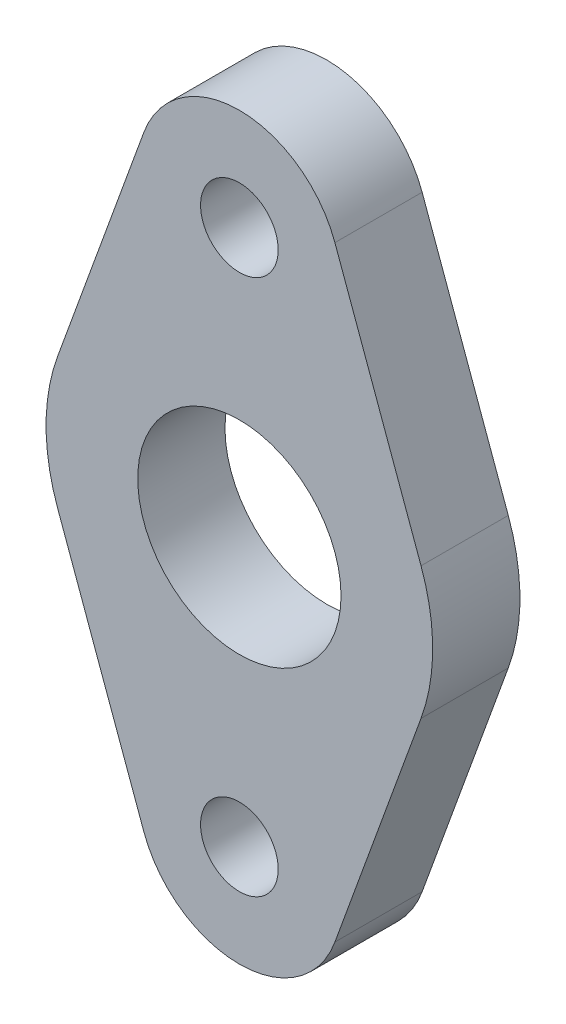
ISO-10303-21;
HEADER;
FILE_DESCRIPTION(('STEP AP214'),'2;1');
FILE_NAME('part.step','',(''),(''),'','','');
FILE_SCHEMA(('AUTOMOTIVE_DESIGN { 1 0 10303 214 1 1 1 1 }'));
ENDSEC;
DATA;
#1=APPLICATION_CONTEXT('core data for automotive mechanical design processes');
#2=APPLICATION_PROTOCOL_DEFINITION('international standard','automotive_design',2000,#1);
#3=PRODUCT_CONTEXT('',#1,'mechanical');
#4=PRODUCT('Part','Part','',(#3));
#5=PRODUCT_RELATED_PRODUCT_CATEGORY('part','',(#4));
#6=PRODUCT_DEFINITION_FORMATION('','',#4);
#7=PRODUCT_DEFINITION_CONTEXT('part definition',#1,'design');
#8=PRODUCT_DEFINITION('design','',#6,#7);
#9=PRODUCT_DEFINITION_SHAPE('','',#8);
#10=(LENGTH_UNIT() NAMED_UNIT(*) SI_UNIT(.MILLI.,.METRE.));
#11=(NAMED_UNIT(*) PLANE_ANGLE_UNIT() SI_UNIT($,.RADIAN.));
#12=(NAMED_UNIT(*) SI_UNIT($,.STERADIAN.) SOLID_ANGLE_UNIT());
#13=UNCERTAINTY_MEASURE_WITH_UNIT(LENGTH_MEASURE(1.E-05),#10,'distance_accuracy_value','');
#14=(GEOMETRIC_REPRESENTATION_CONTEXT(3) GLOBAL_UNCERTAINTY_ASSIGNED_CONTEXT((#13)) GLOBAL_UNIT_ASSIGNED_CONTEXT((#10,
#11,#12)) REPRESENTATION_CONTEXT('',''));
#15=CARTESIAN_POINT('',(0.,0.,0.));
#16=DIRECTION('',(0.,0.,1.));
#17=DIRECTION('',(1.,0.,0.));
#18=AXIS2_PLACEMENT_3D('',#15,#16,#17);
#19=CARTESIAN_POINT('',(0.,-33.5,10.9));
#20=DIRECTION('',(0.,0.,-1.));
#21=DIRECTION('',(-1.,0.,0.));
#22=AXIS2_PLACEMENT_3D('',#19,#20,#21);
#23=CYLINDRICAL_SURFACE('',#22,12.7);
#24=CARTESIAN_POINT('',(0.,-33.5,0.));
#25=DIRECTION('',(0.,0.,1.));
#26=DIRECTION('',(-1.,0.,0.));
#27=AXIS2_PLACEMENT_3D('',#24,#25,#26);
#28=CIRCLE('',#27,12.7);
#29=CARTESIAN_POINT('',(-11.9351548725244,-37.8407462686567,0.));
#30=VERTEX_POINT('',#29);
#31=CARTESIAN_POINT('',(11.9351548725244,-37.8407462686567,0.));
#32=VERTEX_POINT('',#31);
#33=EDGE_CURVE('E140',#30,#32,#28,.T.);
#34=ORIENTED_EDGE('',*,*,#33,.T.);
#35=DIRECTION('',(0.,0.,-1.));
#36=VECTOR('',#35,1.);
#37=CARTESIAN_POINT('',(11.9351548725244,-37.8407462686567,10.9));
#38=LINE('',#37,#36);
#39=CARTESIAN_POINT('',(11.9351548725244,-37.8407462686567,10.9));
#40=VERTEX_POINT('',#39);
#41=EDGE_CURVE('E11',#40,#32,#38,.T.);
#42=ORIENTED_EDGE('',*,*,#41,.F.);
#43=CARTESIAN_POINT('',(0.,-33.5,10.9));
#44=DIRECTION('',(0.,0.,1.));
#45=DIRECTION('',(-1.,0.,0.));
#46=AXIS2_PLACEMENT_3D('',#43,#44,#45);
#47=CIRCLE('',#46,12.7);
#48=CARTESIAN_POINT('',(-11.9351548725244,-37.8407462686567,10.9));
#49=VERTEX_POINT('',#48);
#50=EDGE_CURVE('E151',#49,#40,#47,.T.);
#51=ORIENTED_EDGE('',*,*,#50,.F.);
#52=DIRECTION('',(0.,0.,-1.));
#53=VECTOR('',#52,1.);
#54=CARTESIAN_POINT('',(-11.9351548725244,-37.8407462686567,10.9));
#55=LINE('',#54,#53);
#56=EDGE_CURVE('E135',#49,#30,#55,.T.);
#57=ORIENTED_EDGE('',*,*,#56,.T.);
#58=EDGE_LOOP('',(#34,#42,#51,#57));
#59=FACE_BOUND('',#58,.T.);
#60=ADVANCED_FACE('F39',(#59),#23,.T.);
#61=CARTESIAN_POINT('',(11.9351548725244,-37.8407462686567,10.9));
#62=DIRECTION('',(-0.939775974214519,0.341791044776119,0.));
#63=DIRECTION('',(-0.341791044776119,-0.939775974214519,0.));
#64=AXIS2_PLACEMENT_3D('',#61,#62,#63);
#65=PLANE('',#64);
#66=DIRECTION('',(0.341791044776119,0.939775974214519,0.));
#67=VECTOR('',#66,1.);
#68=CARTESIAN_POINT('',(11.9351548725244,-37.8407462686567,0.));
#69=LINE('',#68,#67);
#70=CARTESIAN_POINT('',(22.6955897772806,-8.25425373134328,0.));
#71=VERTEX_POINT('',#70);
#72=EDGE_CURVE('E139',#32,#71,#69,.T.);
#73=ORIENTED_EDGE('',*,*,#72,.T.);
#74=DIRECTION('',(0.,0.,-1.));
#75=VECTOR('',#74,1.);
#76=CARTESIAN_POINT('',(22.6955897772806,-8.25425373134328,10.9));
#77=LINE('',#76,#75);
#78=CARTESIAN_POINT('',(22.6955897772806,-8.25425373134328,10.9));
#79=VERTEX_POINT('',#78);
#80=EDGE_CURVE('E48',#79,#71,#77,.T.);
#81=ORIENTED_EDGE('',*,*,#80,.F.);
#82=DIRECTION('',(0.341791044776119,0.939775974214519,0.));
#83=VECTOR('',#82,1.);
#84=CARTESIAN_POINT('',(11.9351548725244,-37.8407462686567,10.9));
#85=LINE('',#84,#83);
#86=EDGE_CURVE('E99',#40,#79,#85,.T.);
#87=ORIENTED_EDGE('',*,*,#86,.F.);
#88=ORIENTED_EDGE('',*,*,#41,.T.);
#89=EDGE_LOOP('',(#73,#81,#87,#88));
#90=FACE_BOUND('',#89,.T.);
#91=ADVANCED_FACE('F199',(#90),#65,.F.);
#92=CARTESIAN_POINT('',(0.,0.,10.9));
#93=DIRECTION('',(0.,0.,-1.));
#94=DIRECTION('',(-1.,0.,0.));
#95=AXIS2_PLACEMENT_3D('',#92,#93,#94);
#96=CYLINDRICAL_SURFACE('',#95,24.15);
#97=CARTESIAN_POINT('',(0.,0.,0.));
#98=DIRECTION('',(0.,0.,1.));
#99=DIRECTION('',(1.,0.,0.));
#100=AXIS2_PLACEMENT_3D('',#97,#98,#99);
#101=CIRCLE('',#100,24.15);
#102=CARTESIAN_POINT('',(22.6955897772806,8.25425373134328,0.));
#103=VERTEX_POINT('',#102);
#104=EDGE_CURVE('E142',#71,#103,#101,.T.);
#105=ORIENTED_EDGE('',*,*,#104,.T.);
#106=DIRECTION('',(0.,0.,-1.));
#107=VECTOR('',#106,1.);
#108=CARTESIAN_POINT('',(22.6955897772806,8.25425373134328,10.9));
#109=LINE('',#108,#107);
#110=CARTESIAN_POINT('',(22.6955897772806,8.25425373134328,10.9));
#111=VERTEX_POINT('',#110);
#112=EDGE_CURVE('E158',#111,#103,#109,.T.);
#113=ORIENTED_EDGE('',*,*,#112,.F.);
#114=CARTESIAN_POINT('',(0.,0.,10.9));
#115=DIRECTION('',(0.,0.,1.));
#116=DIRECTION('',(1.,0.,0.));
#117=AXIS2_PLACEMENT_3D('',#114,#115,#116);
#118=CIRCLE('',#117,24.15);
#119=EDGE_CURVE('E288',#79,#111,#118,.T.);
#120=ORIENTED_EDGE('',*,*,#119,.F.);
#121=ORIENTED_EDGE('',*,*,#80,.T.);
#122=EDGE_LOOP('',(#105,#113,#120,#121));
#123=FACE_BOUND('',#122,.T.);
#124=ADVANCED_FACE('F204',(#123),#96,.T.);
#125=CARTESIAN_POINT('',(11.9351548725244,37.8407462686567,10.9));
#126=DIRECTION('',(-0.939775974214519,-0.341791044776119,0.));
#127=DIRECTION('',(0.341791044776119,-0.939775974214519,0.));
#128=AXIS2_PLACEMENT_3D('',#125,#126,#127);
#129=PLANE('',#128);
#130=DIRECTION('',(-0.341791044776119,0.939775974214519,0.));
#131=VECTOR('',#130,1.);
#132=CARTESIAN_POINT('',(11.9351548725244,37.8407462686567,0.));
#133=LINE('',#132,#131);
#134=CARTESIAN_POINT('',(11.9351548725244,37.8407462686567,0.));
#135=VERTEX_POINT('',#134);
#136=EDGE_CURVE('E145',#103,#135,#133,.T.);
#137=ORIENTED_EDGE('',*,*,#136,.T.);
#138=DIRECTION('',(0.,0.,-1.));
#139=VECTOR('',#138,1.);
#140=CARTESIAN_POINT('',(11.9351548725244,37.8407462686567,10.9));
#141=LINE('',#140,#139);
#142=CARTESIAN_POINT('',(11.9351548725244,37.8407462686567,10.9));
#143=VERTEX_POINT('',#142);
#144=EDGE_CURVE('E154',#143,#135,#141,.T.);
#145=ORIENTED_EDGE('',*,*,#144,.F.);
#146=DIRECTION('',(-0.341791044776119,0.939775974214519,0.));
#147=VECTOR('',#146,1.);
#148=CARTESIAN_POINT('',(11.9351548725244,37.8407462686567,10.9));
#149=LINE('',#148,#147);
#150=EDGE_CURVE('E292',#111,#143,#149,.T.);
#151=ORIENTED_EDGE('',*,*,#150,.F.);
#152=ORIENTED_EDGE('',*,*,#112,.T.);
#153=EDGE_LOOP('',(#137,#145,#151,#152));
#154=FACE_BOUND('',#153,.T.);
#155=ADVANCED_FACE('F208',(#154),#129,.F.);
#156=CARTESIAN_POINT('',(0.,33.5,10.9));
#157=DIRECTION('',(0.,0.,-1.));
#158=DIRECTION('',(-1.,0.,0.));
#159=AXIS2_PLACEMENT_3D('',#156,#157,#158);
#160=CYLINDRICAL_SURFACE('',#159,12.7);
#161=CARTESIAN_POINT('',(0.,33.5,0.));
#162=DIRECTION('',(0.,0.,1.));
#163=DIRECTION('',(1.,0.,0.));
#164=AXIS2_PLACEMENT_3D('',#161,#162,#163);
#165=CIRCLE('',#164,12.7);
#166=CARTESIAN_POINT('',(-11.9351548725244,37.8407462686567,0.));
#167=VERTEX_POINT('',#166);
#168=EDGE_CURVE('E148',#135,#167,#165,.T.);
#169=ORIENTED_EDGE('',*,*,#168,.T.);
#170=DIRECTION('',(0.,0.,-1.));
#171=VECTOR('',#170,1.);
#172=CARTESIAN_POINT('',(-11.9351548725244,37.8407462686567,10.9));
#173=LINE('',#172,#171);
#174=CARTESIAN_POINT('',(-11.9351548725244,37.8407462686567,10.9));
#175=VERTEX_POINT('',#174);
#176=EDGE_CURVE('E126',#175,#167,#173,.T.);
#177=ORIENTED_EDGE('',*,*,#176,.F.);
#178=CARTESIAN_POINT('',(0.,33.5,10.9));
#179=DIRECTION('',(0.,0.,1.));
#180=DIRECTION('',(1.,0.,0.));
#181=AXIS2_PLACEMENT_3D('',#178,#179,#180);
#182=CIRCLE('',#181,12.7);
#183=EDGE_CURVE('E118',#143,#175,#182,.T.);
#184=ORIENTED_EDGE('',*,*,#183,.F.);
#185=ORIENTED_EDGE('',*,*,#144,.T.);
#186=EDGE_LOOP('',(#169,#177,#184,#185));
#187=FACE_BOUND('',#186,.T.);
#188=ADVANCED_FACE('F212',(#187),#160,.T.);
#189=CARTESIAN_POINT('',(-11.9351548725244,37.8407462686567,10.9));
#190=DIRECTION('',(0.939775974214519,-0.341791044776119,0.));
#191=DIRECTION('',(0.341791044776119,0.939775974214519,0.));
#192=AXIS2_PLACEMENT_3D('',#189,#190,#191);
#193=PLANE('',#192);
#194=DIRECTION('',(-0.341791044776119,-0.939775974214519,0.));
#195=VECTOR('',#194,1.);
#196=CARTESIAN_POINT('',(-11.9351548725244,37.8407462686567,0.));
#197=LINE('',#196,#195);
#198=CARTESIAN_POINT('',(-22.6955897772806,8.25425373134328,0.));
#199=VERTEX_POINT('',#198);
#200=EDGE_CURVE('E130',#167,#199,#197,.T.);
#201=ORIENTED_EDGE('',*,*,#200,.T.);
#202=DIRECTION('',(0.,0.,-1.));
#203=VECTOR('',#202,1.);
#204=CARTESIAN_POINT('',(-22.6955897772806,8.25425373134328,10.9));
#205=LINE('',#204,#203);
#206=CARTESIAN_POINT('',(-22.6955897772806,8.25425373134328,10.9));
#207=VERTEX_POINT('',#206);
#208=EDGE_CURVE('E123',#207,#199,#205,.T.);
#209=ORIENTED_EDGE('',*,*,#208,.F.);
#210=DIRECTION('',(-0.341791044776119,-0.939775974214519,0.));
#211=VECTOR('',#210,1.);
#212=CARTESIAN_POINT('',(-11.9351548725244,37.8407462686567,10.9));
#213=LINE('',#212,#211);
#214=EDGE_CURVE('E114',#175,#207,#213,.T.);
#215=ORIENTED_EDGE('',*,*,#214,.F.);
#216=ORIENTED_EDGE('',*,*,#176,.T.);
#217=EDGE_LOOP('',(#201,#209,#215,#216));
#218=FACE_BOUND('',#217,.T.);
#219=ADVANCED_FACE('F124',(#218),#193,.F.);
#220=CARTESIAN_POINT('',(0.,0.,10.9));
#221=DIRECTION('',(0.,0.,-1.));
#222=DIRECTION('',(-1.,0.,0.));
#223=AXIS2_PLACEMENT_3D('',#220,#221,#222);
#224=CYLINDRICAL_SURFACE('',#223,24.15);
#225=CARTESIAN_POINT('',(0.,0.,0.));
#226=DIRECTION('',(0.,0.,1.));
#227=DIRECTION('',(1.,0.,0.));
#228=AXIS2_PLACEMENT_3D('',#225,#226,#227);
#229=CIRCLE('',#228,24.15);
#230=CARTESIAN_POINT('',(-22.6955897772806,-8.25425373134328,0.));
#231=VERTEX_POINT('',#230);
#232=EDGE_CURVE('E88',#199,#231,#229,.T.);
#233=ORIENTED_EDGE('',*,*,#232,.T.);
#234=DIRECTION('',(0.,0.,-1.));
#235=VECTOR('',#234,1.);
#236=CARTESIAN_POINT('',(-22.6955897772806,-8.25425373134328,10.9));
#237=LINE('',#236,#235);
#238=CARTESIAN_POINT('',(-22.6955897772806,-8.25425373134328,10.9));
#239=VERTEX_POINT('',#238);
#240=EDGE_CURVE('E129',#239,#231,#237,.T.);
#241=ORIENTED_EDGE('',*,*,#240,.F.);
#242=CARTESIAN_POINT('',(0.,0.,10.9));
#243=DIRECTION('',(0.,0.,1.));
#244=DIRECTION('',(1.,0.,0.));
#245=AXIS2_PLACEMENT_3D('',#242,#243,#244);
#246=CIRCLE('',#245,24.15);
#247=EDGE_CURVE('E116',#207,#239,#246,.T.);
#248=ORIENTED_EDGE('',*,*,#247,.F.);
#249=ORIENTED_EDGE('',*,*,#208,.T.);
#250=EDGE_LOOP('',(#233,#241,#248,#249));
#251=FACE_BOUND('',#250,.T.);
#252=ADVANCED_FACE('F134',(#251),#224,.T.);
#253=CARTESIAN_POINT('',(-11.9351548725244,-37.8407462686567,10.9));
#254=DIRECTION('',(0.939775974214519,0.341791044776119,0.));
#255=DIRECTION('',(-0.341791044776119,0.939775974214519,0.));
#256=AXIS2_PLACEMENT_3D('',#253,#254,#255);
#257=PLANE('',#256);
#258=DIRECTION('',(0.341791044776119,-0.939775974214519,0.));
#259=VECTOR('',#258,1.);
#260=CARTESIAN_POINT('',(-11.9351548725244,-37.8407462686567,0.));
#261=LINE('',#260,#259);
#262=EDGE_CURVE('E95',#231,#30,#261,.T.);
#263=ORIENTED_EDGE('',*,*,#262,.T.);
#264=ORIENTED_EDGE('',*,*,#56,.F.);
#265=DIRECTION('',(0.341791044776119,-0.939775974214519,0.));
#266=VECTOR('',#265,1.);
#267=CARTESIAN_POINT('',(-11.9351548725244,-37.8407462686567,10.9));
#268=LINE('',#267,#266);
#269=EDGE_CURVE('E60',#239,#49,#268,.T.);
#270=ORIENTED_EDGE('',*,*,#269,.F.);
#271=ORIENTED_EDGE('',*,*,#240,.T.);
#272=EDGE_LOOP('',(#263,#264,#270,#271));
#273=FACE_BOUND('',#272,.T.);
#274=ADVANCED_FACE('F188',(#273),#257,.F.);
#275=CARTESIAN_POINT('',(0.,-33.5,10.9));
#276=DIRECTION('',(0.,0.,-1.));
#277=DIRECTION('',(-1.,0.,0.));
#278=AXIS2_PLACEMENT_3D('',#275,#276,#277);
#279=PLANE('',#278);
#280=CARTESIAN_POINT('',(0.,33.5,10.9));
#281=DIRECTION('',(0.,0.,1.));
#282=DIRECTION('',(1.,0.,0.));
#283=AXIS2_PLACEMENT_3D('',#280,#281,#282);
#284=CIRCLE('',#283,4.85);
#285=CARTESIAN_POINT('',(4.85,33.5,10.9));
#286=VERTEX_POINT('',#285);
#287=EDGE_CURVE('E167',#286,#286,#284,.T.);
#288=ORIENTED_EDGE('',*,*,#287,.F.);
#289=EDGE_LOOP('',(#288));
#290=FACE_BOUND('',#289,.T.);
#291=CARTESIAN_POINT('',(0.,-33.5,10.9));
#292=DIRECTION('',(0.,0.,1.));
#293=DIRECTION('',(1.,0.,0.));
#294=AXIS2_PLACEMENT_3D('',#291,#292,#293);
#295=CIRCLE('',#294,4.85);
#296=CARTESIAN_POINT('',(4.85,-33.5,10.9));
#297=VERTEX_POINT('',#296);
#298=EDGE_CURVE('E279',#297,#297,#295,.T.);
#299=ORIENTED_EDGE('',*,*,#298,.F.);
#300=EDGE_LOOP('',(#299));
#301=FACE_BOUND('',#300,.T.);
#302=CARTESIAN_POINT('',(0.,0.,10.9));
#303=DIRECTION('',(0.,0.,1.));
#304=DIRECTION('',(1.,0.,0.));
#305=AXIS2_PLACEMENT_3D('',#302,#303,#304);
#306=CIRCLE('',#305,12.7);
#307=CARTESIAN_POINT('',(12.7,0.,10.9));
#308=VERTEX_POINT('',#307);
#309=EDGE_CURVE('E278',#308,#308,#306,.T.);
#310=ORIENTED_EDGE('',*,*,#309,.F.);
#311=EDGE_LOOP('',(#310));
#312=FACE_BOUND('',#311,.T.);
#313=ORIENTED_EDGE('',*,*,#50,.T.);
#314=ORIENTED_EDGE('',*,*,#86,.T.);
#315=ORIENTED_EDGE('',*,*,#119,.T.);
#316=ORIENTED_EDGE('',*,*,#150,.T.);
#317=ORIENTED_EDGE('',*,*,#183,.T.);
#318=ORIENTED_EDGE('',*,*,#214,.T.);
#319=ORIENTED_EDGE('',*,*,#247,.T.);
#320=ORIENTED_EDGE('',*,*,#269,.T.);
#321=EDGE_LOOP('',(#313,#314,#315,#316,#317,#318,#319,#320));
#322=FACE_BOUND('',#321,.T.);
#323=ADVANCED_FACE('F113',(#290,#301,#312,#322),#279,.F.);
#324=CARTESIAN_POINT('',(0.,-33.5,0.));
#325=DIRECTION('',(0.,0.,-1.));
#326=DIRECTION('',(-1.,0.,0.));
#327=AXIS2_PLACEMENT_3D('',#324,#325,#326);
#328=PLANE('',#327);
#329=CARTESIAN_POINT('',(0.,33.5,0.));
#330=DIRECTION('',(0.,0.,-1.));
#331=DIRECTION('',(-1.,0.,0.));
#332=AXIS2_PLACEMENT_3D('',#329,#330,#331);
#333=CIRCLE('',#332,4.85);
#334=CARTESIAN_POINT('',(-4.85,33.5,0.));
#335=VERTEX_POINT('',#334);
#336=EDGE_CURVE('E45',#335,#335,#333,.T.);
#337=ORIENTED_EDGE('',*,*,#336,.F.);
#338=EDGE_LOOP('',(#337));
#339=FACE_BOUND('',#338,.T.);
#340=CARTESIAN_POINT('',(0.,-33.5,0.));
#341=DIRECTION('',(0.,0.,-1.));
#342=DIRECTION('',(-1.,0.,0.));
#343=AXIS2_PLACEMENT_3D('',#340,#341,#342);
#344=CIRCLE('',#343,4.85);
#345=CARTESIAN_POINT('',(-4.85,-33.5,0.));
#346=VERTEX_POINT('',#345);
#347=EDGE_CURVE('E164',#346,#346,#344,.T.);
#348=ORIENTED_EDGE('',*,*,#347,.F.);
#349=EDGE_LOOP('',(#348));
#350=FACE_BOUND('',#349,.T.);
#351=CARTESIAN_POINT('',(0.,0.,0.));
#352=DIRECTION('',(0.,0.,-1.));
#353=DIRECTION('',(-1.,0.,0.));
#354=AXIS2_PLACEMENT_3D('',#351,#352,#353);
#355=CIRCLE('',#354,12.7);
#356=CARTESIAN_POINT('',(-12.7,0.,0.));
#357=VERTEX_POINT('',#356);
#358=EDGE_CURVE('E162',#357,#357,#355,.T.);
#359=ORIENTED_EDGE('',*,*,#358,.F.);
#360=EDGE_LOOP('',(#359));
#361=FACE_BOUND('',#360,.T.);
#362=ORIENTED_EDGE('',*,*,#33,.F.);
#363=ORIENTED_EDGE('',*,*,#262,.F.);
#364=ORIENTED_EDGE('',*,*,#232,.F.);
#365=ORIENTED_EDGE('',*,*,#200,.F.);
#366=ORIENTED_EDGE('',*,*,#168,.F.);
#367=ORIENTED_EDGE('',*,*,#136,.F.);
#368=ORIENTED_EDGE('',*,*,#104,.F.);
#369=ORIENTED_EDGE('',*,*,#72,.F.);
#370=EDGE_LOOP('',(#362,#363,#364,#365,#366,#367,#368,#369));
#371=FACE_BOUND('',#370,.T.);
#372=ADVANCED_FACE('F176',(#339,#350,#361,#371),#328,.T.);
#373=CARTESIAN_POINT('',(0.,0.,-39.));
#374=DIRECTION('',(0.,0.,1.));
#375=DIRECTION('',(1.,0.,0.));
#376=AXIS2_PLACEMENT_3D('',#373,#374,#375);
#377=CYLINDRICAL_SURFACE('',#376,12.7);
#378=ORIENTED_EDGE('',*,*,#358,.T.);
#379=EDGE_LOOP('',(#378));
#380=FACE_BOUND('',#379,.T.);
#381=ORIENTED_EDGE('',*,*,#309,.T.);
#382=EDGE_LOOP('',(#381));
#383=FACE_BOUND('',#382,.T.);
#384=ADVANCED_FACE('F178',(#380,#383),#377,.F.);
#385=CARTESIAN_POINT('',(0.,-33.5,-39.));
#386=DIRECTION('',(0.,0.,1.));
#387=DIRECTION('',(1.,0.,0.));
#388=AXIS2_PLACEMENT_3D('',#385,#386,#387);
#389=CYLINDRICAL_SURFACE('',#388,4.85);
#390=ORIENTED_EDGE('',*,*,#347,.T.);
#391=EDGE_LOOP('',(#390));
#392=FACE_BOUND('',#391,.T.);
#393=ORIENTED_EDGE('',*,*,#298,.T.);
#394=EDGE_LOOP('',(#393));
#395=FACE_BOUND('',#394,.T.);
#396=ADVANCED_FACE('F254',(#392,#395),#389,.F.);
#397=CARTESIAN_POINT('',(0.,33.5,-39.));
#398=DIRECTION('',(0.,0.,1.));
#399=DIRECTION('',(1.,0.,0.));
#400=AXIS2_PLACEMENT_3D('',#397,#398,#399);
#401=CYLINDRICAL_SURFACE('',#400,4.85);
#402=ORIENTED_EDGE('',*,*,#336,.T.);
#403=EDGE_LOOP('',(#402));
#404=FACE_BOUND('',#403,.T.);
#405=ORIENTED_EDGE('',*,*,#287,.T.);
#406=EDGE_LOOP('',(#405));
#407=FACE_BOUND('',#406,.T.);
#408=ADVANCED_FACE('F175',(#404,#407),#401,.F.);
#409=CLOSED_SHELL('',(#60,#91,#124,#155,#188,#219,#252,#274,#323,#372,#384,#396,#408));
#410=MANIFOLD_SOLID_BREP('B2',#409);
#411=ADVANCED_BREP_SHAPE_REPRESENTATION('',(#18,#410),#14);
#412=SHAPE_DEFINITION_REPRESENTATION(#9,#411);
ENDSEC;
END-ISO-10303-21;
